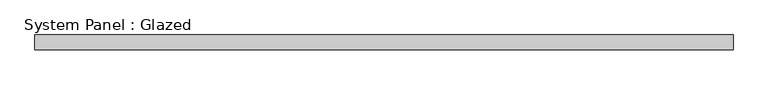
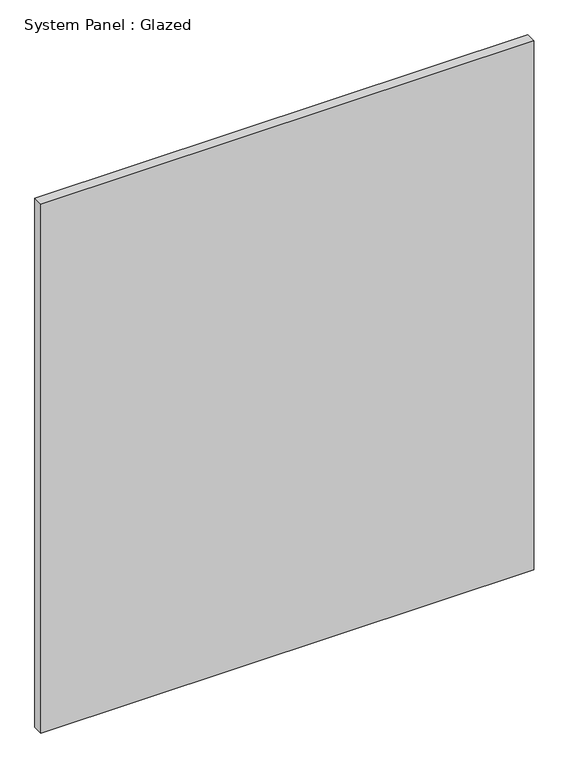
"""IFC4 building model written with IfcOpenShell, lengths in millimetres: plate geometry, System Panel : Glazed."""

from ifc_helpers import new_model, si_unit, origin, origin_with_axes, place, context, project, spatial, polyline, outline, extrude, source, transform, mapped, element, save


def system_panel_glazed_3f3a89de(model_context):
    return source(origin(), model_context, "Body", "SweptSolid", [
        extrude(outline(polyline([(585.0, 24.5), (-585.0, 24.5), (-585.0, 49.5), (585.0, 49.5), (585.0, 24.5)])), origin_with_axes(), (0.0, 0.0, 1.0), 1327.5),
    ])


if __name__ == "__main__":
    model = new_model("IFC4")
    model_context = context("Model", 3, world=origin())
    ifc_project = project(units=[si_unit("LENGTHUNIT", "METRE", prefix="MILLI")], contexts=[model_context])
    site = spatial("IfcSite", under=ifc_project)
    building = spatial("IfcBuilding", under=site)
    placement = place(None, origin())
    system_panel_glazed_shape = system_panel_glazed_3f3a89de(model_context)
    element("IfcPlate", 1, ObjectType="System Panel : Glazed", at=placement, inside=building, context=model_context, shape_type="MappedRepresentation", body=[
        mapped(system_panel_glazed_shape, transform((0.0, 0.0, 0.0), x_axis=(1.0, 0.0, 0.0), y_axis=(0.0, 1.0, 0.0), z_axis=(0.0, 0.0, 1.0))),
    ])
    save(model, "model.ifc")

# Revit data of these elements
# Type "System Panel : Glazed"
#   Construction Type Id = "GSP4R"
#   Analytic Construction = "1/8 in Pilkington single glazing"
#   Visual Light Transmittance = 0.9
#   Solar Heat Gain Coefficient = 0.86
#   Heat Transfer Coefficient (U) = 6.7069 W/(m²·K)
#   Define Thermal Properties by = 1
# Element 1 (IfcPlate, "System Panel : Glazed")
#   Materials on its faces: "Glass"
# Materials
#   "Glass": class "Glass", colour RGB 245 245 243, transparency 1, Description = "Soda Lime Glass", Cost = 0
